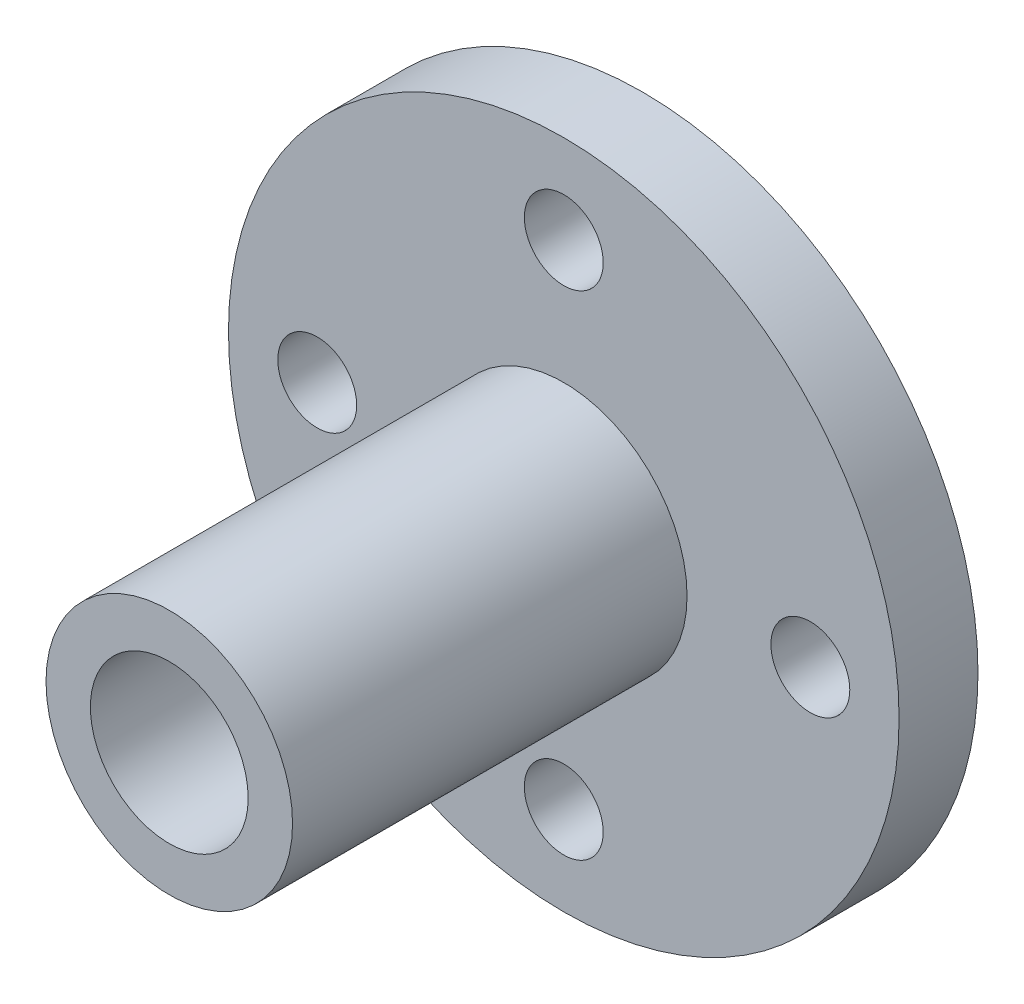
ISO-10303-21;
HEADER;
FILE_DESCRIPTION(('STEP AP214'),'2;1');
FILE_NAME('part.step','',(''),(''),'','','');
FILE_SCHEMA(('AUTOMOTIVE_DESIGN { 1 0 10303 214 1 1 1 1 }'));
ENDSEC;
DATA;
#1=APPLICATION_CONTEXT('core data for automotive mechanical design processes');
#2=APPLICATION_PROTOCOL_DEFINITION('international standard','automotive_design',2000,#1);
#3=PRODUCT_CONTEXT('',#1,'mechanical');
#4=PRODUCT('Part','Part','',(#3));
#5=PRODUCT_RELATED_PRODUCT_CATEGORY('part','',(#4));
#6=PRODUCT_DEFINITION_FORMATION('','',#4);
#7=PRODUCT_DEFINITION_CONTEXT('part definition',#1,'design');
#8=PRODUCT_DEFINITION('design','',#6,#7);
#9=PRODUCT_DEFINITION_SHAPE('','',#8);
#10=(LENGTH_UNIT() NAMED_UNIT(*) SI_UNIT(.MILLI.,.METRE.));
#11=(NAMED_UNIT(*) PLANE_ANGLE_UNIT() SI_UNIT($,.RADIAN.));
#12=(NAMED_UNIT(*) SI_UNIT($,.STERADIAN.) SOLID_ANGLE_UNIT());
#13=UNCERTAINTY_MEASURE_WITH_UNIT(LENGTH_MEASURE(1.E-05),#10,'distance_accuracy_value','');
#14=(GEOMETRIC_REPRESENTATION_CONTEXT(3) GLOBAL_UNCERTAINTY_ASSIGNED_CONTEXT((#13)) GLOBAL_UNIT_ASSIGNED_CONTEXT((#10,
#11,#12)) REPRESENTATION_CONTEXT('',''));
#15=CARTESIAN_POINT('',(0.,0.,0.));
#16=DIRECTION('',(0.,0.,1.));
#17=DIRECTION('',(1.,0.,0.));
#18=AXIS2_PLACEMENT_3D('',#15,#16,#17);
#19=CARTESIAN_POINT('',(0.,0.,4.));
#20=DIRECTION('',(0.,0.,-1.));
#21=DIRECTION('',(-1.,0.,0.));
#22=AXIS2_PLACEMENT_3D('',#19,#20,#21);
#23=CYLINDRICAL_SURFACE('',#22,17.);
#24=CARTESIAN_POINT('',(0.,0.,4.));
#25=DIRECTION('',(0.,0.,1.));
#26=DIRECTION('',(1.,0.,0.));
#27=AXIS2_PLACEMENT_3D('',#24,#25,#26);
#28=CIRCLE('',#27,17.);
#29=CARTESIAN_POINT('',(17.,0.,4.));
#30=VERTEX_POINT('',#29);
#31=EDGE_CURVE('E52',#30,#30,#28,.T.);
#32=ORIENTED_EDGE('',*,*,#31,.F.);
#33=EDGE_LOOP('',(#32));
#34=FACE_BOUND('',#33,.T.);
#35=CARTESIAN_POINT('',(0.,0.,0.));
#36=DIRECTION('',(0.,0.,1.));
#37=DIRECTION('',(1.,0.,0.));
#38=AXIS2_PLACEMENT_3D('',#35,#36,#37);
#39=CIRCLE('',#38,17.);
#40=CARTESIAN_POINT('',(17.,0.,0.));
#41=VERTEX_POINT('',#40);
#42=EDGE_CURVE('E60',#41,#41,#39,.T.);
#43=ORIENTED_EDGE('',*,*,#42,.T.);
#44=EDGE_LOOP('',(#43));
#45=FACE_BOUND('',#44,.T.);
#46=ADVANCED_FACE('F43',(#34,#45),#23,.T.);
#47=CARTESIAN_POINT('',(0.,0.,4.));
#48=DIRECTION('',(0.,0.,1.));
#49=DIRECTION('',(1.,0.,0.));
#50=AXIS2_PLACEMENT_3D('',#47,#48,#49);
#51=PLANE('',#50);
#52=CARTESIAN_POINT('',(0.,12.5,4.));
#53=DIRECTION('',(0.,0.,1.));
#54=DIRECTION('',(1.,0.,0.));
#55=AXIS2_PLACEMENT_3D('',#52,#53,#54);
#56=CIRCLE('',#55,2.);
#57=CARTESIAN_POINT('',(2.,12.5,4.));
#58=VERTEX_POINT('',#57);
#59=EDGE_CURVE('E93',#58,#58,#56,.T.);
#60=ORIENTED_EDGE('',*,*,#59,.F.);
#61=EDGE_LOOP('',(#60));
#62=FACE_BOUND('',#61,.T.);
#63=CARTESIAN_POINT('',(12.5,0.,4.));
#64=DIRECTION('',(0.,0.,1.));
#65=DIRECTION('',(1.,0.,0.));
#66=AXIS2_PLACEMENT_3D('',#63,#64,#65);
#67=CIRCLE('',#66,2.);
#68=CARTESIAN_POINT('',(14.5,0.,4.));
#69=VERTEX_POINT('',#68);
#70=EDGE_CURVE('E84',#69,#69,#67,.T.);
#71=ORIENTED_EDGE('',*,*,#70,.F.);
#72=EDGE_LOOP('',(#71));
#73=FACE_BOUND('',#72,.T.);
#74=CARTESIAN_POINT('',(0.,-12.5,4.));
#75=DIRECTION('',(0.,0.,1.));
#76=DIRECTION('',(1.,0.,0.));
#77=AXIS2_PLACEMENT_3D('',#74,#75,#76);
#78=CIRCLE('',#77,2.);
#79=CARTESIAN_POINT('',(2.,-12.5,4.));
#80=VERTEX_POINT('',#79);
#81=EDGE_CURVE('E76',#80,#80,#78,.T.);
#82=ORIENTED_EDGE('',*,*,#81,.F.);
#83=EDGE_LOOP('',(#82));
#84=FACE_BOUND('',#83,.T.);
#85=CARTESIAN_POINT('',(-12.5,0.,4.));
#86=DIRECTION('',(0.,0.,1.));
#87=DIRECTION('',(1.,0.,0.));
#88=AXIS2_PLACEMENT_3D('',#85,#86,#87);
#89=CIRCLE('',#88,2.);
#90=CARTESIAN_POINT('',(-10.5,0.,4.));
#91=VERTEX_POINT('',#90);
#92=EDGE_CURVE('E75',#91,#91,#89,.T.);
#93=ORIENTED_EDGE('',*,*,#92,.F.);
#94=EDGE_LOOP('',(#93));
#95=FACE_BOUND('',#94,.T.);
#96=CARTESIAN_POINT('',(0.,0.,4.));
#97=DIRECTION('',(0.,0.,1.));
#98=DIRECTION('',(1.,0.,0.));
#99=AXIS2_PLACEMENT_3D('',#96,#97,#98);
#100=CIRCLE('',#99,6.25);
#101=CARTESIAN_POINT('',(6.25,0.,4.));
#102=VERTEX_POINT('',#101);
#103=EDGE_CURVE('E65',#102,#102,#100,.T.);
#104=ORIENTED_EDGE('',*,*,#103,.F.);
#105=EDGE_LOOP('',(#104));
#106=FACE_BOUND('',#105,.T.);
#107=ORIENTED_EDGE('',*,*,#31,.T.);
#108=EDGE_LOOP('',(#107));
#109=FACE_BOUND('',#108,.T.);
#110=ADVANCED_FACE('F124',(#62,#73,#84,#95,#106,#109),#51,.T.);
#111=CARTESIAN_POINT('',(0.,0.,0.));
#112=DIRECTION('',(0.,0.,1.));
#113=DIRECTION('',(1.,0.,0.));
#114=AXIS2_PLACEMENT_3D('',#111,#112,#113);
#115=PLANE('',#114);
#116=CARTESIAN_POINT('',(0.,0.,0.));
#117=DIRECTION('',(0.,0.,1.));
#118=DIRECTION('',(1.,0.,0.));
#119=AXIS2_PLACEMENT_3D('',#116,#117,#118);
#120=CIRCLE('',#119,6.25);
#121=CARTESIAN_POINT('',(6.25,0.,0.));
#122=VERTEX_POINT('',#121);
#123=EDGE_CURVE('E10',#122,#122,#120,.F.);
#124=ORIENTED_EDGE('',*,*,#123,.F.);
#125=EDGE_LOOP('',(#124));
#126=FACE_BOUND('',#125,.T.);
#127=CARTESIAN_POINT('',(0.,12.5,0.));
#128=DIRECTION('',(0.,0.,1.));
#129=DIRECTION('',(1.,0.,0.));
#130=AXIS2_PLACEMENT_3D('',#127,#128,#129);
#131=CIRCLE('',#130,2.);
#132=CARTESIAN_POINT('',(2.,12.5,0.));
#133=VERTEX_POINT('',#132);
#134=EDGE_CURVE('E72',#133,#133,#131,.T.);
#135=ORIENTED_EDGE('',*,*,#134,.T.);
#136=EDGE_LOOP('',(#135));
#137=FACE_BOUND('',#136,.T.);
#138=CARTESIAN_POINT('',(12.5,0.,0.));
#139=DIRECTION('',(0.,0.,1.));
#140=DIRECTION('',(1.,0.,0.));
#141=AXIS2_PLACEMENT_3D('',#138,#139,#140);
#142=CIRCLE('',#141,2.);
#143=CARTESIAN_POINT('',(14.5,0.,0.));
#144=VERTEX_POINT('',#143);
#145=EDGE_CURVE('E86',#144,#144,#142,.T.);
#146=ORIENTED_EDGE('',*,*,#145,.T.);
#147=EDGE_LOOP('',(#146));
#148=FACE_BOUND('',#147,.T.);
#149=CARTESIAN_POINT('',(0.,-12.5,0.));
#150=DIRECTION('',(0.,0.,1.));
#151=DIRECTION('',(1.,0.,0.));
#152=AXIS2_PLACEMENT_3D('',#149,#150,#151);
#153=CIRCLE('',#152,2.);
#154=CARTESIAN_POINT('',(2.,-12.5,0.));
#155=VERTEX_POINT('',#154);
#156=EDGE_CURVE('E85',#155,#155,#153,.T.);
#157=ORIENTED_EDGE('',*,*,#156,.T.);
#158=EDGE_LOOP('',(#157));
#159=FACE_BOUND('',#158,.T.);
#160=CARTESIAN_POINT('',(-12.5,0.,0.));
#161=DIRECTION('',(0.,0.,1.));
#162=DIRECTION('',(1.,0.,0.));
#163=AXIS2_PLACEMENT_3D('',#160,#161,#162);
#164=CIRCLE('',#163,2.);
#165=CARTESIAN_POINT('',(-10.5,0.,0.));
#166=VERTEX_POINT('',#165);
#167=EDGE_CURVE('E73',#166,#166,#164,.T.);
#168=ORIENTED_EDGE('',*,*,#167,.T.);
#169=EDGE_LOOP('',(#168));
#170=FACE_BOUND('',#169,.T.);
#171=ORIENTED_EDGE('',*,*,#42,.F.);
#172=EDGE_LOOP('',(#171));
#173=FACE_BOUND('',#172,.T.);
#174=ADVANCED_FACE('F128',(#126,#137,#148,#159,#170,#173),#115,.F.);
#175=CARTESIAN_POINT('',(0.,0.,24.));
#176=DIRECTION('',(0.,0.,1.));
#177=DIRECTION('',(1.,0.,0.));
#178=AXIS2_PLACEMENT_3D('',#175,#176,#177);
#179=PLANE('',#178);
#180=CARTESIAN_POINT('',(0.,0.,24.));
#181=DIRECTION('',(0.,0.,1.));
#182=DIRECTION('',(1.,0.,0.));
#183=AXIS2_PLACEMENT_3D('',#180,#181,#182);
#184=CIRCLE('',#183,6.25);
#185=CARTESIAN_POINT('',(6.25,0.,24.));
#186=VERTEX_POINT('',#185);
#187=EDGE_CURVE('E62',#186,#186,#184,.T.);
#188=ORIENTED_EDGE('',*,*,#187,.T.);
#189=EDGE_LOOP('',(#188));
#190=FACE_BOUND('',#189,.T.);
#191=CARTESIAN_POINT('',(0.,0.,24.));
#192=DIRECTION('',(0.,0.,1.));
#193=DIRECTION('',(1.,0.,0.));
#194=AXIS2_PLACEMENT_3D('',#191,#192,#193);
#195=CIRCLE('',#194,4.);
#196=CARTESIAN_POINT('',(4.,0.,24.));
#197=VERTEX_POINT('',#196);
#198=EDGE_CURVE('E68',#197,#197,#195,.T.);
#199=ORIENTED_EDGE('',*,*,#198,.F.);
#200=EDGE_LOOP('',(#199));
#201=FACE_BOUND('',#200,.T.);
#202=ADVANCED_FACE('F137',(#190,#201),#179,.T.);
#203=CARTESIAN_POINT('',(0.,0.,24.));
#204=DIRECTION('',(0.,0.,-1.));
#205=DIRECTION('',(-1.,0.,0.));
#206=AXIS2_PLACEMENT_3D('',#203,#204,#205);
#207=CYLINDRICAL_SURFACE('',#206,6.25);
#208=ORIENTED_EDGE('',*,*,#187,.F.);
#209=EDGE_LOOP('',(#208));
#210=FACE_BOUND('',#209,.T.);
#211=ORIENTED_EDGE('',*,*,#103,.T.);
#212=EDGE_LOOP('',(#211));
#213=FACE_BOUND('',#212,.T.);
#214=ADVANCED_FACE('F144',(#210,#213),#207,.T.);
#215=CARTESIAN_POINT('',(0.,0.,24.));
#216=DIRECTION('',(0.,0.,-1.));
#217=DIRECTION('',(-1.,0.,0.));
#218=AXIS2_PLACEMENT_3D('',#215,#216,#217);
#219=CYLINDRICAL_SURFACE('',#218,4.);
#220=ORIENTED_EDGE('',*,*,#198,.T.);
#221=EDGE_LOOP('',(#220));
#222=FACE_BOUND('',#221,.T.);
#223=CARTESIAN_POINT('',(0.,0.,4.));
#224=DIRECTION('',(0.,0.,1.));
#225=DIRECTION('',(1.,0.,0.));
#226=AXIS2_PLACEMENT_3D('',#223,#224,#225);
#227=CIRCLE('',#226,4.);
#228=CARTESIAN_POINT('',(4.,0.,4.));
#229=VERTEX_POINT('',#228);
#230=EDGE_CURVE('E47',#229,#229,#227,.F.);
#231=ORIENTED_EDGE('',*,*,#230,.T.);
#232=EDGE_LOOP('',(#231));
#233=FACE_BOUND('',#232,.T.);
#234=ADVANCED_FACE('F211',(#222,#233),#219,.F.);
#235=ORIENTED_EDGE('',*,*,#230,.F.);
#236=EDGE_LOOP('',(#235));
#237=FACE_BOUND('',#236,.T.);
#238=ADVANCED_FACE('F135',(#237),#51,.T.);
#239=CARTESIAN_POINT('',(-12.5,0.,0.));
#240=DIRECTION('',(0.,0.,1.));
#241=DIRECTION('',(1.,0.,0.));
#242=AXIS2_PLACEMENT_3D('',#239,#240,#241);
#243=CYLINDRICAL_SURFACE('',#242,2.);
#244=ORIENTED_EDGE('',*,*,#167,.F.);
#245=EDGE_LOOP('',(#244));
#246=FACE_BOUND('',#245,.T.);
#247=ORIENTED_EDGE('',*,*,#92,.T.);
#248=EDGE_LOOP('',(#247));
#249=FACE_BOUND('',#248,.T.);
#250=ADVANCED_FACE('F193',(#246,#249),#243,.F.);
#251=CARTESIAN_POINT('',(0.,-12.5,0.));
#252=DIRECTION('',(0.,0.,1.));
#253=DIRECTION('',(1.,0.,0.));
#254=AXIS2_PLACEMENT_3D('',#251,#252,#253);
#255=CYLINDRICAL_SURFACE('',#254,2.);
#256=ORIENTED_EDGE('',*,*,#156,.F.);
#257=EDGE_LOOP('',(#256));
#258=FACE_BOUND('',#257,.T.);
#259=ORIENTED_EDGE('',*,*,#81,.T.);
#260=EDGE_LOOP('',(#259));
#261=FACE_BOUND('',#260,.T.);
#262=ADVANCED_FACE('F182',(#258,#261),#255,.F.);
#263=CARTESIAN_POINT('',(12.5,0.,0.));
#264=DIRECTION('',(0.,0.,1.));
#265=DIRECTION('',(1.,0.,0.));
#266=AXIS2_PLACEMENT_3D('',#263,#264,#265);
#267=CYLINDRICAL_SURFACE('',#266,2.);
#268=ORIENTED_EDGE('',*,*,#145,.F.);
#269=EDGE_LOOP('',(#268));
#270=FACE_BOUND('',#269,.T.);
#271=ORIENTED_EDGE('',*,*,#70,.T.);
#272=EDGE_LOOP('',(#271));
#273=FACE_BOUND('',#272,.T.);
#274=ADVANCED_FACE('F118',(#270,#273),#267,.F.);
#275=CARTESIAN_POINT('',(0.,12.5,0.));
#276=DIRECTION('',(0.,0.,1.));
#277=DIRECTION('',(1.,0.,0.));
#278=AXIS2_PLACEMENT_3D('',#275,#276,#277);
#279=CYLINDRICAL_SURFACE('',#278,2.);
#280=ORIENTED_EDGE('',*,*,#134,.F.);
#281=EDGE_LOOP('',(#280));
#282=FACE_BOUND('',#281,.T.);
#283=ORIENTED_EDGE('',*,*,#59,.T.);
#284=EDGE_LOOP('',(#283));
#285=FACE_BOUND('',#284,.T.);
#286=ADVANCED_FACE('F112',(#282,#285),#279,.F.);
#287=CARTESIAN_POINT('',(0.,0.,-1.));
#288=DIRECTION('',(0.,0.,-1.));
#289=DIRECTION('',(-1.,0.,0.));
#290=AXIS2_PLACEMENT_3D('',#287,#288,#289);
#291=PLANE('',#290);
#292=CARTESIAN_POINT('',(0.,0.,-1.));
#293=DIRECTION('',(0.,0.,-1.));
#294=DIRECTION('',(-1.,0.,0.));
#295=AXIS2_PLACEMENT_3D('',#292,#293,#294);
#296=CIRCLE('',#295,6.25);
#297=CARTESIAN_POINT('',(-6.25,0.,-1.));
#298=VERTEX_POINT('',#297);
#299=EDGE_CURVE('E77',#298,#298,#296,.T.);
#300=ORIENTED_EDGE('',*,*,#299,.T.);
#301=EDGE_LOOP('',(#300));
#302=FACE_BOUND('',#301,.T.);
#303=CARTESIAN_POINT('',(0.,0.,-1.));
#304=DIRECTION('',(0.,0.,-1.));
#305=DIRECTION('',(-1.,0.,0.));
#306=AXIS2_PLACEMENT_3D('',#303,#304,#305);
#307=CIRCLE('',#306,4.);
#308=CARTESIAN_POINT('',(-4.,0.,-1.));
#309=VERTEX_POINT('',#308);
#310=EDGE_CURVE('E98',#309,#309,#307,.T.);
#311=ORIENTED_EDGE('',*,*,#310,.F.);
#312=EDGE_LOOP('',(#311));
#313=FACE_BOUND('',#312,.T.);
#314=ADVANCED_FACE('F107',(#302,#313),#291,.T.);
#315=CARTESIAN_POINT('',(0.,0.,-1.));
#316=DIRECTION('',(0.,0.,1.));
#317=DIRECTION('',(1.,0.,0.));
#318=AXIS2_PLACEMENT_3D('',#315,#316,#317);
#319=CYLINDRICAL_SURFACE('',#318,6.25);
#320=ORIENTED_EDGE('',*,*,#299,.F.);
#321=EDGE_LOOP('',(#320));
#322=FACE_BOUND('',#321,.T.);
#323=ORIENTED_EDGE('',*,*,#123,.T.);
#324=EDGE_LOOP('',(#323));
#325=FACE_BOUND('',#324,.T.);
#326=ADVANCED_FACE('F109',(#322,#325),#319,.T.);
#327=CARTESIAN_POINT('',(0.,0.,-1.));
#328=DIRECTION('',(0.,0.,1.));
#329=DIRECTION('',(1.,0.,0.));
#330=AXIS2_PLACEMENT_3D('',#327,#328,#329);
#331=CYLINDRICAL_SURFACE('',#330,4.);
#332=ORIENTED_EDGE('',*,*,#310,.T.);
#333=EDGE_LOOP('',(#332));
#334=FACE_BOUND('',#333,.T.);
#335=CARTESIAN_POINT('',(0.,0.,0.));
#336=DIRECTION('',(0.,0.,-1.));
#337=DIRECTION('',(-1.,0.,0.));
#338=AXIS2_PLACEMENT_3D('',#335,#336,#337);
#339=CIRCLE('',#338,4.);
#340=CARTESIAN_POINT('',(-4.,0.,0.));
#341=VERTEX_POINT('',#340);
#342=EDGE_CURVE('E97',#341,#341,#339,.T.);
#343=ORIENTED_EDGE('',*,*,#342,.F.);
#344=EDGE_LOOP('',(#343));
#345=FACE_BOUND('',#344,.T.);
#346=ADVANCED_FACE('F104',(#334,#345),#331,.F.);
#347=ORIENTED_EDGE('',*,*,#342,.T.);
#348=EDGE_LOOP('',(#347));
#349=FACE_BOUND('',#348,.T.);
#350=ADVANCED_FACE('F143',(#349),#115,.F.);
#351=CLOSED_SHELL('',(#46,#110,#174,#202,#214,#234,#238,#250,#262,#274,#286,#314,#326,#346,#350));
#352=MANIFOLD_SOLID_BREP('B2',#351);
#353=ADVANCED_BREP_SHAPE_REPRESENTATION('',(#18,#352),#14);
#354=SHAPE_DEFINITION_REPRESENTATION(#9,#353);
ENDSEC;
END-ISO-10303-21;
